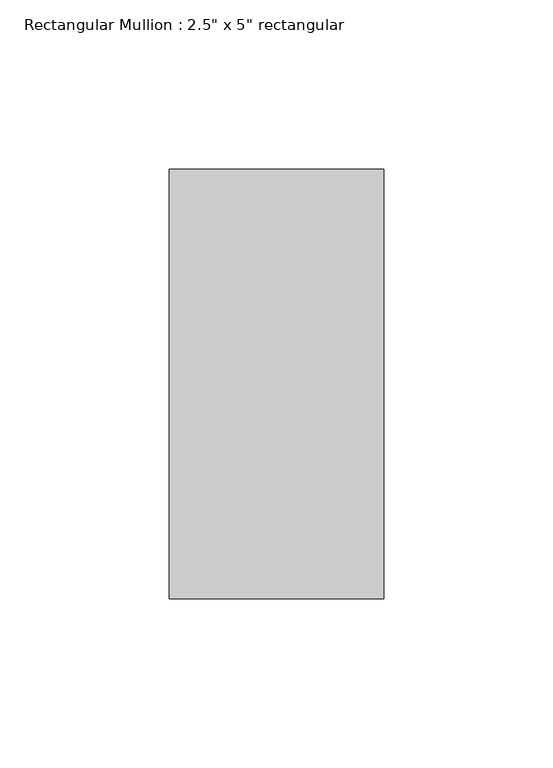
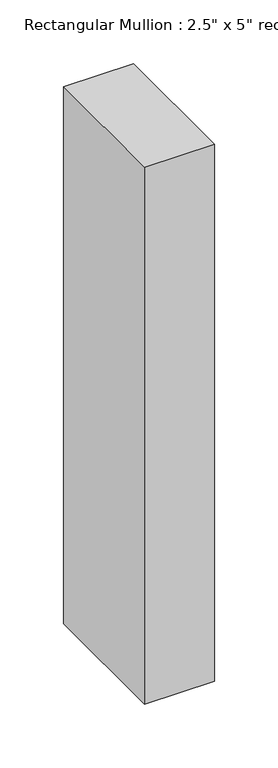
"""IFC4 building model written with IfcOpenShell, lengths in millimetres: member geometry."""

from ifc_helpers import new_model, si_unit, frame, origin, place, context, project, spatial, polyline, outline, extrude, source, transform, mapped, element, save


def member_0b7646a3(model_context):
    return source(origin(), model_context, "Body", "SweptSolid", [
        extrude(outline(polyline([(0.0, 63.5), (0.0, -63.5), (-63.5, -63.5), (-63.5, 63.5), (0.0, 63.5)])), frame((0.0, 0.0, -514.35), z_axis=(0.0, 0.0, 1.0), x_axis=(1.0, 0.0, 0.0)), (0.0, 0.0, 1.0), 514.35),
    ])


if __name__ == "__main__":
    model = new_model("IFC4")
    model_context = context("Model", 3, world=origin())
    ifc_project = project(units=[si_unit("LENGTHUNIT", "METRE", prefix="MILLI")], contexts=[model_context])
    site = spatial("IfcSite", under=ifc_project)
    building = spatial("IfcBuilding", under=site)
    placement = place(None, origin())
    member_shape = member_0b7646a3(model_context)
    element("IfcMember", 1, ObjectType="Rectangular Mullion : 2.5\" x 5\" rectangular", at=placement, inside=building, context=model_context, shape_type="MappedRepresentation", body=[
        mapped(member_shape, transform((0.0, 0.0, 0.0), x_axis=(1.0, 0.0, 0.0), y_axis=(0.0, 1.0, 0.0), z_axis=(0.0, 0.0, 1.0))),
    ])
    save(model, "model.ifc")

# Revit data of these elements
# Type "Rectangular Mullion : 2.5\" x 5\" rectangular"
#   built-in parameter 1007304 = 0.416667 (stored number, unit not read)
#   built-in parameter 1007301 = 0.104167 (stored number, unit not read)
#   built-in parameter 1007300 = 0.104167 (stored number, unit not read)
